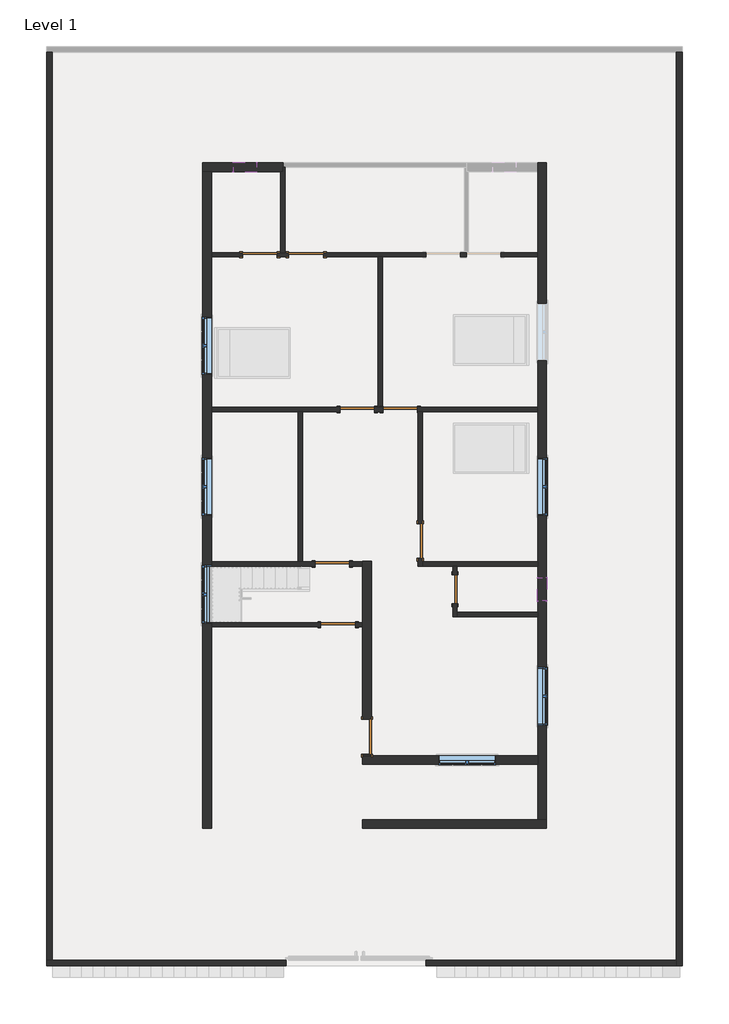
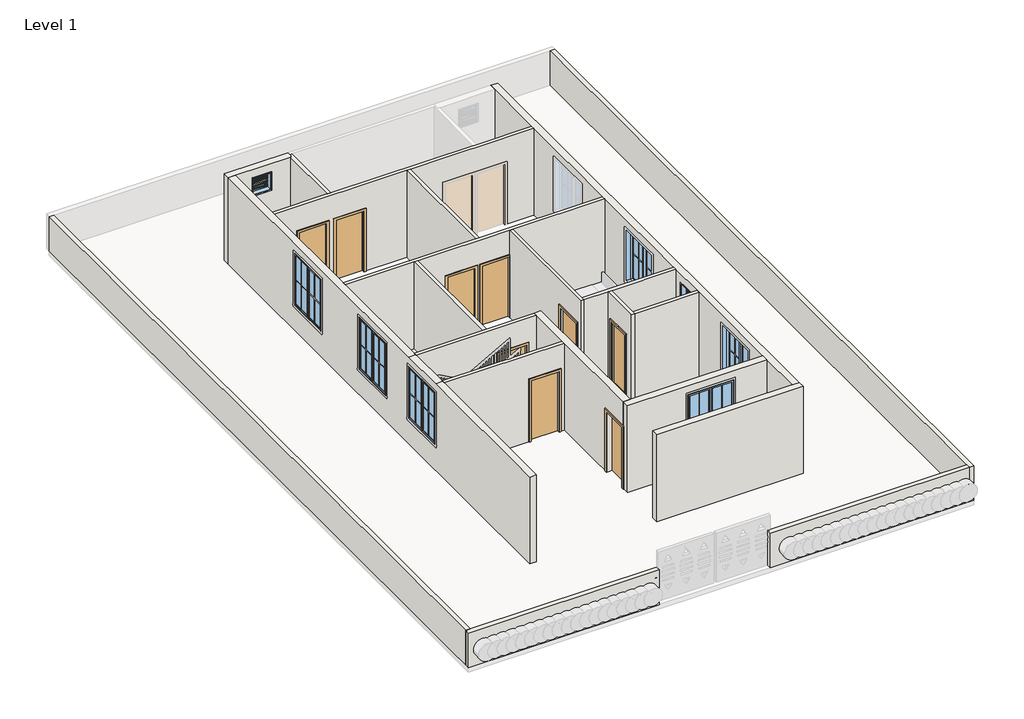
# One storey, part 1 of 3: 21 walls, 9 doors, 8 windows.
"""IFC4 building model written with IfcOpenShell, lengths in millimetres."""

from ifc_helpers import new_model, si_unit, frame, origin, origin_with_axes, place, context, project, spatial, polyline, outline, extrude, faceted_brep, transform, mapped, element, save
from components import door_78caadf7, single_flush_door_3_e5f9f3c4, single_flush_door_3_305aa2a5, single_flush_door_3_0ca8825f, window_casement_double_win_5_f93960c7, window_f2d8fef0

model = new_model("IFC4")

# Units and contexts
model_context = context("Model", 3, world=origin())
ifc_project = project(units=[si_unit("LENGTHUNIT", "METRE", prefix="MILLI")], contexts=[model_context])

# Site, building, storey
site = spatial("IfcSite", under=ifc_project)
building = spatial("IfcBuilding", under=site)
storey = spatial("IfcBuildingStorey", under=building, Name="Level 1", Elevation=0.0)

# Doors
placement = place(None, origin())
door_shape = door_78caadf7(model_context)
element("IfcDoor", 1, ObjectType="Single-Flush : DOOR 2'6\"", at=placement, inside=storey, context=model_context, shape_type="MappedRepresentation", body=[
    mapped(door_shape, transform((860.2379845, -2779.6065691, 0.0), x_axis=(0.0, 1.0, 0.0), y_axis=(-1.0, 0.0, 0.0), z_axis=(0.0, 0.0, 1.0))),
])
single_flush_door_3_shape = single_flush_door_3_e5f9f3c4(model_context)
element("IfcDoor", 2, ObjectType="Single-Flush : DOOR 3'", at=placement, inside=storey, context=model_context, shape_type="MappedRepresentation", body=[
    mapped(single_flush_door_3_shape, transform((-54.1620155, -1503.2565691, 0.0), x_axis=(0.0, -1.0, 0.0), y_axis=(1.0, 0.0, 0.0), z_axis=(0.0, 0.0, 1.0))),
])
element("IfcDoor", 3, ObjectType="Single-Flush : DOOR 3'", at=placement, inside=storey, context=model_context, shape_type="MappedRepresentation", body=[
    mapped(single_flush_door_3_shape, transform((-1717.8620155, 1963.8434309, 0.0), x_axis=(1.0, 0.0, 0.0), y_axis=(0.0, 1.0, 0.0), z_axis=(0.0, 0.0, 1.0))),
])
element("IfcDoor", 4, ObjectType="Single-Flush : DOOR 3'", at=placement, inside=storey, context=model_context, shape_type="MappedRepresentation", body=[
    mapped(single_flush_door_3_shape, transform((-2371.9120155, -2112.8565691, 0.0), x_axis=(1.0, 0.0, 0.0), y_axis=(0.0, 1.0, 0.0), z_axis=(0.0, 0.0, 1.0))),
])
element("IfcDoor", 5, ObjectType="Single-Flush : DOOR 3'", at=placement, inside=storey, context=model_context, shape_type="MappedRepresentation", body=[
    mapped(single_flush_door_3_shape, transform((-2219.5120155, -3713.0565691, 0.0), x_axis=(1.0, 0.0, 0.0), y_axis=(0.0, 1.0, 0.0), z_axis=(0.0, 0.0, 1.0))),
])
element("IfcDoor", 6, ObjectType="Single-Flush : DOOR 3'", at=placement, inside=storey, context=model_context, shape_type="MappedRepresentation", body=[
    mapped(single_flush_door_3_shape, transform((-4283.2620155, 6040.5434309, 0.0), x_axis=(1.0, 0.0, 0.0), y_axis=(0.0, 1.0, 0.0), z_axis=(0.0, 0.0, 1.0))),
])
single_flush_door_3_2_shape = single_flush_door_3_305aa2a5(model_context)
element("IfcDoor", 7, ObjectType="Single-Flush : DOOR 3'", at=placement, inside=storey, context=model_context, shape_type="MappedRepresentation", body=[
    mapped(single_flush_door_3_2_shape, transform((-581.2120155, 1963.8434309, 0.0), x_axis=(-1.0, 0.0, 0.0), y_axis=(0.0, -1.0, 0.0), z_axis=(0.0, 0.0, 1.0))),
])
element("IfcDoor", 8, ObjectType="Single-Flush : DOOR 3'", at=placement, inside=storey, context=model_context, shape_type="MappedRepresentation", body=[
    mapped(single_flush_door_3_2_shape, transform((-3064.0620155, 6040.5434309, 0.0), x_axis=(-1.0, 0.0, 0.0), y_axis=(0.0, -1.0, 0.0), z_axis=(0.0, 0.0, 1.0))),
])
single_flush_door_3_3_shape = single_flush_door_3_0ca8825f(model_context)
element("IfcDoor", 9, ObjectType="Single-Flush : DOOR 3'", at=placement, inside=storey, context=model_context, shape_type="MappedRepresentation", body=[
    mapped(single_flush_door_3_3_shape, transform((-1457.5120155, -6665.8065691, 0.0), x_axis=(0.0, -1.0, 0.0), y_axis=(1.0, 0.0, 0.0), z_axis=(0.0, 0.0, 1.0))),
])

# Walls
element("IfcWall", 10, ObjectType="CMD 6\"", at=placement, inside=storey, context=model_context, shape_type="Brep", body=[
    faceted_brep([(6701.4726148, 11374.8947978, 0.0), (6701.4726148, -12551.9052022, 0.0), (6701.4726148, -12704.3052022, 0.0), (6701.4726148, -12704.3052022, 1219.2), (6701.4726148, -12551.9052022, 1219.2), (6701.4726148, 11374.8947978, 1219.2), (6853.8726148, 11374.8947978, 0.0), (6853.8726148, 11374.8947978, 1219.2), (6853.8726148, -12704.3052022, 1219.2), (6853.8726148, -12704.3052022, 0.0)], [[[0, 1, 2, 3, 4, 5]], [[6, 7, 8, 9]], [[2, 1, 0, 6, 9]], [[5, 4, 3, 8, 7]], [[0, 5, 7, 6]], [[3, 2, 9, 8]]]),
])
element("IfcWall", 11, ObjectType="CMD 6\"", at=placement, inside=storey, context=model_context, shape_type="SweptSolid", body=[
    extrude(outline(polyline([(102.2665881, -12551.9052022), (6701.4726148, -12551.9052022), (6701.4726148, -12704.3052022), (102.2665881, -12704.3052022), (102.2665881, -12551.9052022)])), origin_with_axes(), (0.0, 0.0, 1.0), 1219.2),
])
element("IfcWall", 12, ObjectType="CMD 6\"", at=placement, inside=storey, context=model_context, shape_type="SweptSolid", body=[
    extrude(outline(polyline([(-9757.7273852, 11374.8947978), (-9757.7273852, -12551.9052022), (-9910.1273852, -12551.9052022), (-9910.1273852, 11374.8947978), (-9757.7273852, 11374.8947978)])), origin_with_axes(), (0.0, 0.0, 1.0), 1219.2),
])
element("IfcWall", 13, ObjectType="CMD 6\"", at=placement, inside=storey, context=model_context, shape_type="Brep", body=[
    faceted_brep([(-3585.5273852, -12551.9052022, 0.0), (-9757.7273852, -12551.9052022, 0.0), (-9910.1273852, -12551.9052022, 0.0), (-9910.1273852, -12551.9052022, 1219.2), (-9757.7273852, -12551.9052022, 1219.2), (-3585.5273852, -12551.9052022, 1219.2), (-3585.5273852, -12704.3052022, 0.0), (-3585.5273852, -12704.3052022, 1219.2), (-9910.1273852, -12704.3052022, 1219.2), (-9910.1273852, -12704.3052022, 0.0)], [[[0, 1, 2, 3, 4, 5]], [[6, 7, 8, 9]], [[2, 1, 0, 6, 9]], [[5, 4, 3, 8, 7]], [[0, 5, 7, 6]], [[3, 2, 9, 8]]]),
])
element("IfcWall", 14, ObjectType="WALL 4.5\"", at=placement, inside=storey, context=model_context, shape_type="SweptSolid", body=[
    extrude(outline(polyline([(-3730.8120155, 6097.6934309), (-3730.8120155, 8231.2934309), (-3673.6620155, 8231.2934309), (-3673.6620155, 8345.5934309), (-3616.5120155, 8345.5934309), (-3616.5120155, 6097.6934309), (-3730.8120155, 6097.6934309)])), origin_with_axes(), (0.0, 0.0, 1.0), 3048.0),
])
element("IfcWall", 15, ObjectType="WALL 4.5\"", at=placement, inside=storey, context=model_context, shape_type="Brep", body=[
    faceted_brep([(1165.0379845, 6097.6934309, 2133.6), (1165.0379845, 6097.6934309, 0.0), (1107.8879845, 6097.6934309, 0.0), (1012.6379845, 6097.6934309, 0.0), (1012.6379845, 6097.6934309, 2133.6), (98.2379845, 6097.6934309, 2133.6), (98.2379845, 6097.6934309, 0.0), (-2606.8620155, 6097.6934309, 0.0), (-2606.8620155, 6097.6934309, 2133.6), (-3521.2620155, 6097.6934309, 2133.6), (-3521.2620155, 6097.6934309, 0.0), (-3616.5120155, 6097.6934309, 0.0), (-3730.8120155, 6097.6934309, 0.0), (-3826.0620155, 6097.6934309, 0.0), (-3826.0620155, 6097.6934309, 2133.6), (-4740.4620155, 6097.6934309, 2133.6), (-4740.4620155, 6097.6934309, 0.0), (-5559.6120155, 6097.6934309, 0.0), (-5559.6120155, 6097.6934309, 3048.0), (-3730.8120155, 6097.6934309, 3048.0), (-3616.5120155, 6097.6934309, 3048.0), (1107.8879845, 6097.6934309, 3048.0), (1222.1879845, 6097.6934309, 3048.0), (3050.9879845, 6097.6934309, 3048.0), (3050.9879845, 6097.6934309, 0.0), (2079.4379845, 6097.6934309, 0.0), (2079.4379845, 6097.6934309, 2133.6), (1012.6379845, 5983.3934309, 0.0), (1165.0379845, 5983.3934309, 0.0), (1165.0379845, 5983.3934309, 2133.6), (2079.4379845, 5983.3934309, 2133.6), (2079.4379845, 5983.3934309, 0.0), (3050.9879845, 5983.3934309, 0.0), (3050.9879845, 5983.3934309, 3048.0), (-1051.1120155, 5983.3934309, 3048.0), (-1165.4120155, 5983.3934309, 3048.0), (-5559.6120155, 5983.3934309, 3048.0), (-5559.6120155, 5983.3934309, 0.0), (-4740.4620155, 5983.3934309, 0.0), (-4740.4620155, 5983.3934309, 2133.6), (-3826.0620155, 5983.3934309, 2133.6), (-3826.0620155, 5983.3934309, 0.0), (-3521.2620155, 5983.3934309, 0.0), (-3521.2620155, 5983.3934309, 2133.6), (-2606.8620155, 5983.3934309, 2133.6), (-2606.8620155, 5983.3934309, 0.0), (-1165.4120155, 5983.3934309, 0.0), (-1051.1120155, 5983.3934309, 0.0), (98.2379845, 5983.3934309, 0.0), (98.2379845, 5983.3934309, 2133.6), (1012.6379845, 5983.3934309, 2133.6)], [[[0, 1, 2, 3, 4, 5, 6, 7, 8, 9, 10, 11, 12, 13, 14, 15, 16, 17, 18, 19, 20, 21, 22, 23, 24, 25, 26]], [[27, 28, 29, 30, 31, 32, 33, 34, 35, 36, 37, 38, 39, 40, 41, 42, 43, 44, 45, 46, 47, 48, 49, 50]], [[38, 37, 17, 16]], [[13, 12, 11, 10, 42, 41]], [[48, 47, 46, 45, 7, 6]], [[25, 24, 32, 31]], [[3, 2, 1, 28, 27]], [[18, 17, 37, 36]], [[24, 23, 33, 32]], [[14, 13, 41, 40]], [[15, 14, 40, 39]], [[16, 15, 39, 38]], [[43, 42, 10, 9]], [[44, 43, 9, 8]], [[45, 44, 8, 7]], [[4, 3, 27, 50]], [[5, 4, 50, 49]], [[6, 5, 49, 48]], [[29, 28, 1, 0]], [[30, 29, 0, 26]], [[31, 30, 26, 25]], [[23, 22, 21, 20, 19, 18, 36, 35, 34, 33]]]),
])
element("IfcWall", 16, ObjectType="WALL 4.5\"", at=placement, inside=storey, context=model_context, shape_type="SweptSolid", body=[
    extrude(outline(polyline([(-1165.4120155, 2020.9934309), (-1165.4120155, 5983.3934309), (-1051.1120155, 5983.3934309), (-1051.1120155, 2020.9934309), (-1165.4120155, 2020.9934309)])), origin_with_axes(), (0.0, 0.0, 1.0), 3048.0),
])
element("IfcWall", 17, ObjectType="WALL 4.5\"", at=placement, inside=storey, context=model_context, shape_type="Brep", body=[
    faceted_brep([(-1260.6620155, 1906.6934309, 2133.6), (-1260.6620155, 1906.6934309, 0.0), (-1038.4120155, 1906.6934309, 0.0), (-1038.4120155, 1906.6934309, 2133.6), (-124.0120155, 1906.6934309, 2133.6), (-124.0120155, 1906.6934309, 0.0), (-111.3120155, 1906.6934309, 0.0), (2.9879845, 1906.6934309, 0.0), (3050.9879845, 1906.6934309, 0.0), (3050.9879845, 1906.6934309, 3048.0), (2.9879845, 1906.6934309, 3048.0), (-111.3120155, 1906.6934309, 3048.0), (-3159.3120155, 1906.6934309, 3048.0), (-3273.6120155, 1906.6934309, 3048.0), (-5559.6120155, 1906.6934309, 3048.0), (-5559.6120155, 1906.6934309, 0.0), (-3273.6120155, 1906.6934309, 0.0), (-3159.3120155, 1906.6934309, 0.0), (-2175.0620155, 1906.6934309, 0.0), (-2175.0620155, 1906.6934309, 2133.6), (-1038.4120155, 2020.9934309, 0.0), (-1051.1120155, 2020.9934309, 0.0), (-1165.4120155, 2020.9934309, 0.0), (-1260.6620155, 2020.9934309, 0.0), (-1260.6620155, 2020.9934309, 2133.6), (-2175.0620155, 2020.9934309, 2133.6), (-2175.0620155, 2020.9934309, 0.0), (-5559.6120155, 2020.9934309, 0.0), (-5559.6120155, 2020.9934309, 3048.0), (-1165.4120155, 2020.9934309, 3048.0), (-1051.1120155, 2020.9934309, 3048.0), (3050.9879845, 2020.9934309, 3048.0), (3050.9879845, 2020.9934309, 0.0), (-124.0120155, 2020.9934309, 0.0), (-124.0120155, 2020.9934309, 2133.6), (-1038.4120155, 2020.9934309, 2133.6)], [[[0, 1, 2, 3, 4, 5, 6, 7, 8, 9, 10, 11, 12, 13, 14, 15, 16, 17, 18, 19]], [[20, 21, 22, 23, 24, 25, 26, 27, 28, 29, 30, 31, 32, 33, 34, 35]], [[33, 32, 8, 7, 6, 5]], [[2, 1, 23, 22, 21, 20]], [[18, 17, 16, 15, 27, 26]], [[15, 14, 28, 27]], [[9, 8, 32, 31]], [[3, 2, 20, 35]], [[4, 3, 35, 34]], [[5, 4, 34, 33]], [[24, 23, 1, 0]], [[25, 24, 0, 19]], [[26, 25, 19, 18]], [[14, 13, 12, 11, 10, 9, 31, 30, 29, 28]]]),
])
element("IfcWall", 18, ObjectType="WALL 4.5\"", at=placement, inside=storey, context=model_context, shape_type="SweptSolid", body=[
    extrude(outline(polyline([(-3273.6120155, -2032.8465691), (-3273.6120155, 1906.6934309), (-3159.3120155, 1906.6934309), (-3159.3120155, -2032.8465691), (-3273.6120155, -2032.8465691)])), origin_with_axes(), (0.0, 0.0, 1.0), 3048.0),
])
element("IfcWall", 19, ObjectType="WALL 4.5\"", at=placement, inside=storey, context=model_context, shape_type="SweptSolid", body=[
    extrude(outline(polyline([(2133.6, -1914.7120155), (0.0, -1914.7120155), (0.0, -1571.8120155), (3048.0, -1571.8120155), (3048.0, -5559.6120155), (0.0, -5559.6120155), (0.0, -2829.1120155), (2133.6, -2829.1120155), (2133.6, -1914.7120155)])), frame((0.0, -2170.0065691, 0.0), z_axis=(0.0, 1.0, 0.0), x_axis=(0.0, 0.0, 1.0)), (0.0, 0.0, 1.0), 114.3),
])
element("IfcWall", 20, ObjectType="WALL 4.5\"", at=placement, inside=storey, context=model_context, shape_type="SweptSolid", body=[
    extrude(outline(polyline([(2133.6, -1762.3120155), (0.0, -1762.3120155), (0.0, -1571.8120155), (3048.0, -1571.8120155), (3048.0, -5559.6120155), (0.0, -5559.6120155), (0.0, -2676.7120155), (2133.6, -2676.7120155), (2133.6, -1762.3120155)])), frame((0.0, -3770.2065691, 0.0), z_axis=(0.0, 1.0, 0.0), x_axis=(0.0, 0.0, 1.0)), (0.0, 0.0, 1.0), 114.3),
])
element("IfcWall", 21, ObjectType="WALL 4.5\"", at=placement, inside=storey, context=model_context, shape_type="Brep", body=[
    faceted_brep([(-111.3120155, -1960.4565691, 2133.6), (-111.3120155, -1960.4565691, 0.0), (-111.3120155, -2170.0065691, 0.0), (-111.3120155, -2170.0065691, 3048.0), (-111.3120155, 1906.6934309, 3048.0), (-111.3120155, 1906.6934309, 0.0), (-111.3120155, -1046.0565691, 0.0), (-111.3120155, -1046.0565691, 2133.6), (2.9879845, -2170.0065691, 0.0), (2.9879845, -2055.7065691, 0.0), (2.9879845, -1960.4565691, 0.0), (2.9879845, -1960.4565691, 2133.6), (2.9879845, -1046.0565691, 2133.6), (2.9879845, -1046.0565691, 0.0), (2.9879845, 1906.6934309, 0.0), (2.9879845, 1906.6934309, 3048.0), (2.9879845, -2055.7065691, 3048.0), (2.9879845, -2170.0065691, 3048.0)], [[[0, 1, 2, 3, 4, 5, 6, 7]], [[8, 9, 10, 11, 12, 13, 14, 15, 16, 17]], [[6, 5, 14, 13]], [[2, 1, 10, 9, 8]], [[5, 4, 15, 14]], [[3, 2, 8, 17]], [[11, 10, 1, 0]], [[12, 11, 0, 7]], [[13, 12, 7, 6]], [[4, 3, 17, 16, 15]]]),
])
element("IfcWall", 22, ObjectType="WALL 4.5\"", at=placement, inside=storey, context=model_context, shape_type="Brep", body=[
    faceted_brep([(2.9879845, -2170.0065691, 0.0), (803.0879845, -2170.0065691, 0.0), (917.3879845, -2170.0065691, 0.0), (3050.9879845, -2170.0065691, 0.0), (3050.9879845, -2170.0065691, 3048.0), (917.3879845, -2170.0065691, 3048.0), (803.0879845, -2170.0065691, 3048.0), (2.9879845, -2170.0065691, 3048.0), (2.9879845, -2055.7065691, 0.0), (2.9879845, -2055.7065691, 3048.0), (3050.9879845, -2055.7065691, 3048.0), (3050.9879845, -2055.7065691, 0.0)], [[[0, 1, 2, 3, 4, 5, 6, 7]], [[8, 9, 10, 11]], [[3, 2, 1, 0, 8, 11]], [[0, 7, 9, 8]], [[4, 3, 11, 10]], [[7, 6, 5, 4, 10, 9]]]),
])
element("IfcWall", 23, ObjectType="WALL 4.5\"", at=placement, inside=storey, context=model_context, shape_type="Brep", body=[
    faceted_brep([(803.0879845, -2170.0065691, 0.0), (803.0879845, -2398.6065691, 0.0), (803.0879845, -2398.6065691, 2133.6), (803.0879845, -3160.6065691, 2133.6), (803.0879845, -3160.6065691, 0.0), (803.0879845, -3503.5065691, 0.0), (803.0879845, -3503.5065691, 3048.0), (803.0879845, -2170.0065691, 3048.0), (917.3879845, -2398.6065691, 2133.6), (917.3879845, -2398.6065691, 0.0), (917.3879845, -2170.0065691, 0.0), (917.3879845, -2170.0065691, 3048.0), (917.3879845, -3389.2065691, 3048.0), (917.3879845, -3503.5065691, 3048.0), (917.3879845, -3503.5065691, 0.0), (917.3879845, -3389.2065691, 0.0), (917.3879845, -3160.6065691, 0.0), (917.3879845, -3160.6065691, 2133.6)], [[[0, 1, 2, 3, 4, 5, 6, 7]], [[8, 9, 10, 11, 12, 13, 14, 15, 16, 17]], [[10, 9, 1, 0]], [[16, 15, 14, 5, 4]], [[0, 7, 11, 10]], [[6, 5, 14, 13]], [[2, 1, 9, 8]], [[3, 2, 8, 17]], [[4, 3, 17, 16]], [[7, 6, 13, 12, 11]]]),
])
element("IfcWall", 24, ObjectType="WALL 4.5\"", at=placement, inside=storey, context=model_context, shape_type="SweptSolid", body=[
    extrude(outline(polyline([(917.3879845, -3389.2065691), (3050.9879845, -3389.2065691), (3050.9879845, -3503.5065691), (917.3879845, -3503.5065691), (917.3879845, -3389.2065691)])), origin_with_axes(), (0.0, 0.0, 1.0), 3048.0),
])
element("IfcWall", 25, ObjectType="WALL 9\"", at=placement, inside=storey, context=model_context, shape_type="Brep", body=[
    faceted_brep([(-3673.6620155, 8459.8934309, 0.0), (-5788.2120155, 8459.8934309, 0.0), (-5788.2120155, 8459.8934309, 3048.0), (-3673.6620155, 8459.8934309, 3048.0), (-4978.5870155, 8459.8934309, 2743.2), (-4978.5870155, 8459.8934309, 2133.6), (-4368.9870155, 8459.8934309, 2133.6), (-4368.9870155, 8459.8934309, 2743.2), (-3673.6620155, 8231.2934309, 0.0), (-3673.6620155, 8231.2934309, 3048.0), (-3730.8120155, 8231.2934309, 3048.0), (-5559.6120155, 8231.2934309, 3048.0), (-5788.2120155, 8231.2934309, 3048.0), (-5788.2120155, 8231.2934309, 0.0), (-5559.6120155, 8231.2934309, 0.0), (-3730.8120155, 8231.2934309, 0.0), (-4978.5870155, 8231.2934309, 2743.2), (-4368.9870155, 8231.2934309, 2743.2), (-4368.9870155, 8231.2934309, 2133.6), (-4978.5870155, 8231.2934309, 2133.6), (-3673.6620155, 8345.5934309, 0.0), (-3673.6620155, 8345.5934309, 3048.0)], [[[0, 1, 2, 3], [4, 5, 6, 7]], [[8, 9, 10, 11, 12, 13, 14, 15], [16, 17, 18, 19]], [[1, 0, 20, 8, 15, 14, 13]], [[0, 3, 21, 9, 8, 20]], [[2, 1, 13, 12]], [[5, 4, 16, 19]], [[6, 5, 19, 18]], [[7, 6, 18, 17]], [[4, 7, 17, 16]], [[3, 2, 12, 11, 10, 9, 21]]]),
])
element("IfcWall", 26, ObjectType="WALL 9\"", at=placement, inside=storey, context=model_context, shape_type="Brep", body=[
    faceted_brep([(-5788.2120155, 8231.2934309, 0.0), (-5788.2120155, -9078.8065691, 0.0), (-5788.2120155, -9078.8065691, 3048.0), (-5788.2120155, -3674.9565691, 3048.0), (-5788.2120155, -2150.9565691, 3048.0), (-5788.2120155, 8231.2934309, 3048.0), (-5788.2120155, 4402.2434309, 2743.2), (-5788.2120155, 2878.2434309, 2743.2), (-5788.2120155, 2878.2434309, 914.4), (-5788.2120155, 4402.2434309, 914.4), (-5788.2120155, -2150.9565691, 2743.2), (-5788.2120155, -3674.9565691, 2743.2), (-5788.2120155, -3674.9565691, 914.4), (-5788.2120155, -2150.9565691, 914.4), (-5788.2120155, 687.4934309, 2743.2), (-5788.2120155, -836.5065691, 2743.2), (-5788.2120155, -836.5065691, 914.4), (-5788.2120155, 687.4934309, 914.4), (-5559.6120155, 8231.2934309, 0.0), (-5559.6120155, 8231.2934309, 3048.0), (-5559.6120155, 6097.6934309, 3048.0), (-5559.6120155, 5983.3934309, 3048.0), (-5559.6120155, 2020.9934309, 3048.0), (-5559.6120155, 1906.6934309, 3048.0), (-5559.6120155, -2055.7065691, 3048.0), (-5559.6120155, -2150.9565691, 3048.0), (-5559.6120155, -2170.0065691, 3048.0), (-5559.6120155, -3655.9065691, 3048.0), (-5559.6120155, -3674.9565691, 3048.0), (-5559.6120155, -3770.2065691, 3048.0), (-5559.6120155, -9078.8065691, 3048.0), (-5559.6120155, -9078.8065691, 0.0), (-5559.6120155, -3770.2065691, 0.0), (-5559.6120155, -3655.9065691, 0.0), (-5559.6120155, -2170.0065691, 0.0), (-5559.6120155, -2055.7065691, 0.0), (-5559.6120155, 1906.6934309, 0.0), (-5559.6120155, 2020.9934309, 0.0), (-5559.6120155, 5983.3934309, 0.0), (-5559.6120155, 6097.6934309, 0.0), (-5559.6120155, 4402.2434309, 2743.2), (-5559.6120155, 4402.2434309, 914.4), (-5559.6120155, 2878.2434309, 914.4), (-5559.6120155, 2878.2434309, 2743.2), (-5559.6120155, -2150.9565691, 2743.2), (-5559.6120155, -2150.9565691, 914.4), (-5559.6120155, -3674.9565691, 914.4), (-5559.6120155, -3674.9565691, 2743.2), (-5559.6120155, 687.4934309, 2743.2), (-5559.6120155, 687.4934309, 914.4), (-5559.6120155, -836.5065691, 914.4), (-5559.6120155, -836.5065691, 2743.2)], [[[0, 1, 2, 3, 4, 5], [6, 7, 8, 9], [10, 11, 12, 13], [14, 15, 16, 17]], [[18, 19, 20, 21, 22, 23, 24, 25, 26, 27, 28, 29, 30, 31, 32, 33, 34, 35, 36, 37, 38, 39], [40, 41, 42, 43], [44, 45, 46, 47], [48, 49, 50, 51]], [[1, 0, 18, 39, 38, 37, 36, 35, 34, 33, 32, 31]], [[2, 1, 31, 30]], [[0, 5, 19, 18]], [[41, 40, 6, 9]], [[42, 41, 9, 8]], [[43, 42, 8, 7]], [[40, 43, 7, 6]], [[45, 44, 10, 13]], [[46, 45, 13, 12]], [[47, 46, 12, 11]], [[44, 47, 11, 10]], [[49, 48, 14, 17]], [[50, 49, 17, 16]], [[51, 50, 16, 15]], [[48, 51, 15, 14]], [[4, 3, 28, 27, 26, 25]], [[3, 2, 30, 29, 28]], [[5, 4, 25, 24, 23, 22, 21, 20, 19]]]),
])
element("IfcWall", 27, ObjectType="WALL 9\"", at=placement, inside=storey, context=model_context, shape_type="Brep", body=[
    faceted_brep([(-1571.8120155, -9078.8065691, 0.0), (3279.5879845, -9078.8065691, 0.0), (3279.5879845, -9078.8065691, 3048.0), (-1571.8120155, -9078.8065691, 3048.0), (-1571.8120155, -8850.2065691, 0.0), (-1571.8120155, -8850.2065691, 3048.0), (3050.9879845, -8850.2065691, 3048.0), (3279.5879845, -8850.2065691, 3048.0), (3279.5879845, -8850.2065691, 0.0), (3050.9879845, -8850.2065691, 0.0)], [[[0, 1, 2, 3]], [[4, 5, 6, 7, 8, 9]], [[1, 0, 4, 9, 8]], [[0, 3, 5, 4]], [[2, 1, 8, 7]], [[3, 2, 7, 6, 5]]]),
])
element("IfcWall", 28, ObjectType="WALL 9\"", at=placement, inside=storey, context=model_context, shape_type="Brep", body=[
    faceted_brep([(3279.5879845, -8850.2065691, 0.0), (3279.5879845, 8459.8934309, 0.0), (3279.5879845, 8459.8934309, 3048.0), (3279.5879845, -8850.2065691, 3048.0), (3279.5879845, 3240.1934309, 2743.2), (3279.5879845, 4764.1934309, 2743.2), (3279.5879845, 4764.1934309, 914.4), (3279.5879845, 3240.1934309, 914.4), (3279.5879845, -836.5065691, 2743.2), (3279.5879845, 687.4934309, 2743.2), (3279.5879845, 687.4934309, 914.4), (3279.5879845, -836.5065691, 914.4), (3279.5879845, -6361.0065691, 2743.2), (3279.5879845, -4837.0065691, 2743.2), (3279.5879845, -4837.0065691, 914.4), (3279.5879845, -6361.0065691, 914.4), (3279.5879845, -2474.8065691, 2743.2), (3279.5879845, -2474.8065691, 2133.6), (3279.5879845, -3084.4065691, 2133.6), (3279.5879845, -3084.4065691, 2743.2), (3050.9879845, -8850.2065691, 0.0), (3050.9879845, -8850.2065691, 3048.0), (3050.9879845, -7389.7065691, 3048.0), (3050.9879845, -7161.1065691, 3048.0), (3050.9879845, -3503.5065691, 3048.0), (3050.9879845, -3389.2065691, 3048.0), (3050.9879845, -2170.0065691, 3048.0), (3050.9879845, -2055.7065691, 3048.0), (3050.9879845, 1906.6934309, 3048.0), (3050.9879845, 2020.9934309, 3048.0), (3050.9879845, 5983.3934309, 3048.0), (3050.9879845, 6097.6934309, 3048.0), (3050.9879845, 8231.2934309, 3048.0), (3050.9879845, 8459.8934309, 3048.0), (3050.9879845, 8459.8934309, 0.0), (3050.9879845, 8231.2934309, 0.0), (3050.9879845, 6097.6934309, 0.0), (3050.9879845, 5983.3934309, 0.0), (3050.9879845, 2020.9934309, 0.0), (3050.9879845, 1906.6934309, 0.0), (3050.9879845, -2055.7065691, 0.0), (3050.9879845, -2170.0065691, 0.0), (3050.9879845, -3389.2065691, 0.0), (3050.9879845, -3503.5065691, 0.0), (3050.9879845, -7161.1065691, 0.0), (3050.9879845, -7389.7065691, 0.0), (3050.9879845, 3240.1934309, 2743.2), (3050.9879845, 3240.1934309, 914.4), (3050.9879845, 4764.1934309, 914.4), (3050.9879845, 4764.1934309, 2743.2), (3050.9879845, -836.5065691, 2743.2), (3050.9879845, -836.5065691, 914.4), (3050.9879845, 687.4934309, 914.4), (3050.9879845, 687.4934309, 2743.2), (3050.9879845, -6361.0065691, 2743.2), (3050.9879845, -6361.0065691, 914.4), (3050.9879845, -4837.0065691, 914.4), (3050.9879845, -4837.0065691, 2743.2), (3050.9879845, -2474.8065691, 2743.2), (3050.9879845, -3084.4065691, 2743.2), (3050.9879845, -3084.4065691, 2133.6), (3050.9879845, -2474.8065691, 2133.6)], [[[0, 1, 2, 3], [4, 5, 6, 7], [8, 9, 10, 11], [12, 13, 14, 15], [16, 17, 18, 19]], [[20, 21, 22, 23, 24, 25, 26, 27, 28, 29, 30, 31, 32, 33, 34, 35, 36, 37, 38, 39, 40, 41, 42, 43, 44, 45], [46, 47, 48, 49], [50, 51, 52, 53], [54, 55, 56, 57], [58, 59, 60, 61]], [[1, 0, 20, 45, 44, 43, 42, 41, 40, 39, 38, 37, 36, 35, 34]], [[0, 3, 21, 20]], [[2, 1, 34, 33]], [[47, 46, 4, 7]], [[48, 47, 7, 6]], [[49, 48, 6, 5]], [[46, 49, 5, 4]], [[51, 50, 8, 11]], [[52, 51, 11, 10]], [[53, 52, 10, 9]], [[50, 53, 9, 8]], [[55, 54, 12, 15]], [[56, 55, 15, 14]], [[57, 56, 14, 13]], [[54, 57, 13, 12]], [[17, 16, 58, 61]], [[18, 17, 61, 60]], [[19, 18, 60, 59]], [[16, 19, 59, 58]], [[3, 2, 33, 32, 31, 30, 29, 28, 27, 26, 25, 24, 23, 22, 21]]]),
])
element("IfcWall", 29, ObjectType="WALL 9\"", at=placement, inside=storey, context=model_context, shape_type="Brep", body=[
    faceted_brep([(3050.9879845, -7161.1065691, 0.0), (-1343.2120155, -7161.1065691, 0.0), (-1571.8120155, -7161.1065691, 0.0), (-1571.8120155, -7161.1065691, 3048.0), (-1343.2120155, -7161.1065691, 3048.0), (3050.9879845, -7161.1065691, 3048.0), (422.0879845, -7161.1065691, 2743.2), (422.0879845, -7161.1065691, 914.4), (1946.0879845, -7161.1065691, 914.4), (1946.0879845, -7161.1065691, 2743.2), (3050.9879845, -7389.7065691, 0.0), (3050.9879845, -7389.7065691, 3048.0), (-1571.8120155, -7389.7065691, 3048.0), (-1571.8120155, -7389.7065691, 0.0), (422.0879845, -7389.7065691, 2743.2), (1946.0879845, -7389.7065691, 2743.2), (1946.0879845, -7389.7065691, 914.4), (422.0879845, -7389.7065691, 914.4)], [[[0, 1, 2, 3, 4, 5], [6, 7, 8, 9]], [[10, 11, 12, 13], [14, 15, 16, 17]], [[2, 1, 0, 10, 13]], [[0, 5, 11, 10]], [[3, 2, 13, 12]], [[7, 6, 14, 17]], [[8, 7, 17, 16]], [[9, 8, 16, 15]], [[6, 9, 15, 14]], [[5, 4, 3, 12, 11]]]),
])
element("IfcWall", 30, ObjectType="WALL 9\"", at=placement, inside=storey, context=model_context, shape_type="Brep", body=[
    faceted_brep([(-1343.2120155, -7161.1065691, 0.0), (-1343.2120155, -7123.0065691, 0.0), (-1343.2120155, -7123.0065691, 2133.6), (-1343.2120155, -6208.6065691, 2133.6), (-1343.2120155, -6208.6065691, 0.0), (-1343.2120155, -2032.8465691, 0.0), (-1343.2120155, -2032.8465691, 3048.0), (-1343.2120155, -7161.1065691, 3048.0), (-1571.8120155, -7123.0065691, 2133.6), (-1571.8120155, -7123.0065691, 0.0), (-1571.8120155, -7161.1065691, 0.0), (-1571.8120155, -7161.1065691, 3048.0), (-1571.8120155, -3770.2065691, 3048.0), (-1571.8120155, -3655.9065691, 3048.0), (-1571.8120155, -2170.0065691, 3048.0), (-1571.8120155, -2055.7065691, 3048.0), (-1571.8120155, -2032.8465691, 3048.0), (-1571.8120155, -2032.8465691, 0.0), (-1571.8120155, -2055.7065691, 0.0), (-1571.8120155, -2170.0065691, 0.0), (-1571.8120155, -3655.9065691, 0.0), (-1571.8120155, -3770.2065691, 0.0), (-1571.8120155, -6208.6065691, 0.0), (-1571.8120155, -6208.6065691, 2133.6)], [[[0, 1, 2, 3, 4, 5, 6, 7]], [[8, 9, 10, 11, 12, 13, 14, 15, 16, 17, 18, 19, 20, 21, 22, 23]], [[10, 9, 1, 0]], [[22, 21, 20, 19, 18, 17, 5, 4]], [[6, 5, 17, 16]], [[0, 7, 11, 10]], [[2, 1, 9, 8]], [[3, 2, 8, 23]], [[4, 3, 23, 22]], [[7, 6, 16, 15, 14, 13, 12, 11]]]),
])

# Windows
window_casement_double_win_5_shape = window_casement_double_win_5_f93960c7(model_context)
element("IfcWindow", 31, ObjectType="Window-Casement-Double : WIN 5'", at=placement, inside=storey, context=model_context, shape_type="MappedRepresentation", body=[
    mapped(window_casement_double_win_5_shape, transform((-5673.9120155, 3640.2434309, 0.0), x_axis=(0.0, 1.0, 0.0), y_axis=(-1.0, 0.0, 0.0), z_axis=(0.0, 0.0, 1.0))),
])
element("IfcWindow", 32, ObjectType="Window-Casement-Double : WIN 5'", at=placement, inside=storey, context=model_context, shape_type="MappedRepresentation", body=[
    mapped(window_casement_double_win_5_shape, transform((3165.2879845, -74.5065691, 0.0), x_axis=(0.0, -1.0, 0.0), y_axis=(1.0, 0.0, 0.0), z_axis=(0.0, 0.0, 1.0))),
])
element("IfcWindow", 33, ObjectType="Window-Casement-Double : WIN 5'", at=placement, inside=storey, context=model_context, shape_type="MappedRepresentation", body=[
    mapped(window_casement_double_win_5_shape, transform((3165.2879845, -5599.0065691, 0.0), x_axis=(0.0, -1.0, 0.0), y_axis=(1.0, 0.0, 0.0), z_axis=(0.0, 0.0, 1.0))),
])
element("IfcWindow", 34, ObjectType="Window-Casement-Double : WIN 5'", at=placement, inside=storey, context=model_context, shape_type="MappedRepresentation", body=[
    mapped(window_casement_double_win_5_shape, transform((1184.0879845, -7275.4065691, 0.0), x_axis=(-1.0, 0.0, 0.0), y_axis=(0.0, -1.0, 0.0), z_axis=(0.0, 0.0, 1.0))),
])
element("IfcWindow", 35, ObjectType="Window-Casement-Double : WIN 5'", at=placement, inside=storey, context=model_context, shape_type="MappedRepresentation", body=[
    mapped(window_casement_double_win_5_shape, transform((-5673.9120155, -2912.9565691, 0.0), x_axis=(0.0, 1.0, 0.0), y_axis=(-1.0, 0.0, 0.0), z_axis=(0.0, 0.0, 1.0))),
])
element("IfcWindow", 36, ObjectType="Window-Casement-Double : WIN 5'", at=placement, inside=storey, context=model_context, shape_type="MappedRepresentation", body=[
    mapped(window_casement_double_win_5_shape, transform((-5673.9120155, -74.5065691, 0.0), x_axis=(0.0, 1.0, 0.0), y_axis=(-1.0, 0.0, 0.0), z_axis=(0.0, 0.0, 1.0))),
])
window_shape = window_f2d8fef0(model_context)
element("IfcWindow", 37, ObjectType="Window-Louvers : 24\" x 24\"", at=placement, inside=storey, context=model_context, shape_type="MappedRepresentation", body=[
    mapped(window_shape, transform((-4673.7870155, 8351.9434309, 1219.2), x_axis=(1.0, 0.0, 0.0), y_axis=(0.0, 1.0, 0.0), z_axis=(0.0, 0.0, 1.0))),
])
element("IfcWindow", 38, ObjectType="Window-Louvers : 24\" x 24\"", at=placement, inside=storey, context=model_context, shape_type="MappedRepresentation", body=[
    mapped(window_shape, transform((3171.6379845, -2779.6065691, 1219.2), x_axis=(0.0, -1.0, 0.0), y_axis=(1.0, 0.0, 0.0), z_axis=(0.0, 0.0, 1.0))),
])

save(model, "model.ifc")

# Revit data of these elements
# Type "Single-Flush : DOOR 2'6\""
#   Type Mark = "10"
#   Construction Type Id = "MDOOR"
#   Assembly Code = "C1020"
#   Analytic Construction = "Metal"
#   Thickness = 0' - 2"
#   Heat Transfer Coefficient (U) = 0.651978 BTU/(h·ft²·°F)
#   Height = 7' - 0"
#   Trim Projection Ext = 0' - 1"
#   Trim Projection Int = 0' - 1"
#   Trim Width = 0' - 3"
#   Width = 2' - 6"
#   Define Thermal Properties by = 1
#   Door Material = Door - Panel
#   Frame Material = Door - Frame
#   Visual Light Transmittance = 0
#   Solar Heat Gain Coefficient = 0
#   Function = (empty or 0)
#   Wall Closure = (empty or 0)
# Type "Single-Flush : DOOR 3'"
#   Type Mark = "9"
#   Construction Type Id = "MDOOR"
#   Assembly Code = "C1020"
#   Analytic Construction = "Metal"
#   Thickness = 0' - 2"
#   Heat Transfer Coefficient (U) = 0.651978 BTU/(h·ft²·°F)
#   Height = 7' - 0"
#   Trim Projection Ext = 0' - 1"
#   Trim Projection Int = 0' - 1"
#   Trim Width = 0' - 3"
#   Width = 3' - 0"
#   Define Thermal Properties by = 1
#   Door Material = Door - Panel
#   Frame Material = Door - Frame
#   Visual Light Transmittance = 0
#   Solar Heat Gain Coefficient = 0
#   Function = (empty or 0)
#   Wall Closure = (empty or 0)
# Type "CMD 6\""
#   Assembly Code = "B2010"
#   Layers, outside or top first: 0' - 6" no material (function 1)
# Type "WALL 4.5\""
#   Assembly Code = "B2010"
#   Layers, outside or top first: 0' - 4 1/2" no material (function 1)
# Type "WALL 9\""
#   Assembly Code = "B2010"
#   Layers, outside or top first: 0' - 9" no material (function 1)
# Type "Window-Casement-Double : WIN 5'"
#   Type Mark = "18"
#   Fire Rating = "0.5h"
#   Assembly Code = "B2020100"
#   Analytic Construction = "Double glazing - domestic"
#   Frame Extension [instance default] = 0' - 0 1/4"
#   Window Inset [instance default] = 0' - 0"
#   Wall Thickness [instance default] = 0' - 6"
#   Interior Wall Closure [instance default] = 0' - 2 1/4"
#   Half Width = 2' - 6"
#   Visual Light Transmittance = 0.81
#   Thermal Resistance (R) = 1.8146 (h·ft²·°F)/BTU
#   Solar Heat Gain Coefficient = 0.76
#   Rough Width = 5' - 0 1/2"
#   Rough Height = 6' - 0 1/2"
#   Height = 6' - 0"
#   Heat Transfer Coefficient (U) = 0.5511 BTU/(h·ft²·°F)
#   Exterior Wall Closure [instance default] = 0' - 1 1/4"
#   Extension Jamb [instance default] = 0' - 2 1/4"
#   Default Sill Height = 3' - 0"
#   Width = 5' - 0"
#   Muntin Visibility = yes
#   Interior Trim Visibility [instance default] = yes
#   Exterior Trim Visibility [instance default] = yes
#   Extension Jamb Visibility [instance default] = yes
#   Interior Trim Material = Wood - Stained
#   Muntin Pattern = Muntin Pattern_2x2 : Muntin Pattern_2x2
#   Interior Trim = Trim-Window-Interior-Flat : Picture Frame
#   Interior Frame Material = Wood - Stained
#   Glass Panel Material = Glass
#   Exterior Trim Material = Clad - White
#   Exterior Trim = Trim-Window-Exterior-Flat : with Sill
#   Exterior Frame Material = Clad - White
#   Wall Closure = (empty or 0)
# Type "Window-Louvers : 24\" x 24\""
#   Type Mark = "19"
#   Construction Type Id = "GSP4R"
#   Assembly Code = "B20"
#   Analytic Construction = "1/8 in Pilkington single glazing"
#   Visual Light Transmittance = 0.9
#   Thermal Resistance (R) = 1.53941 (h·ft²·°F)/BTU
#   Solar Heat Gain Coefficient = 0.78
#   Max Height = 1' - 11.74264"
#   Height = 2' - 0"
#   Heat Transfer Coefficient (U) = 0.6496 BTU/(h·ft²·°F)
#   Blade Width [instance default] = 1' - 10 1/2"
#   Blade Vertical Thickness = 0' - 0.35355"
#   Blade Thickness = 0' - 0 1/4"
#   Blade Spacing = 0' - 1 1/2"
#   Blade Height = 0' - 1.85355"
#   Blade Depth = 0' - 3"
#   Blade Angle = 45.00°
#   Default Sill Height = 3' - 0"
#   Trim Projection_Exterior = 0' - 0 1/2"
#   Trim Projection_Interior = 0' - 0 1/2"
#   Trim Width_Exterior = 0' - 1 1/2"
#   Trim Width_Interior = 0' - 1 1/2"
#   Width = 2' - 0"
#   Max Blade Count = 12
#   Define Thermal Properties by = 1
#   Blade Count = 12
#   Frame Material = Birch
#   Louver Material = Birch
#   Trim Exterior Material = Birch
#   Trim Interior Material = Birch
#   Wall Closure = (empty or 0)
# Element 1 (IfcDoor, "Single-Flush : DOOR 2'6\"")
#   Phase Created = New Construction
#   Materials on its faces: "Door - Frame", "Door - Panel"
# Elements 2, 3, 4, 5, 6, 7, 8, 9 (IfcDoor, "Single-Flush : DOOR 3'")
#   Phase Created = New Construction
#   Materials on its faces: "Door - Frame", "Door - Panel"
# Elements 10, 13 (IfcWall, "CMD 6\"")
#   Top Offset = 0' - 0"
#   Base Offset = 0' - 0"
#   Unconnected Height = 4' - 0"
#   wall height = 4' - 0"
#   Phase Created = New Construction
#   Base Constraint = Level 1
#   Materials on its faces: "Copper", "Default Wall"
# Elements 11, 12 (IfcWall, "CMD 6\"")
#   Top Offset = 0' - 0"
#   Base Offset = 0' - 0"
#   Unconnected Height = 4' - 0"
#   wall height = 4' - 0"
#   Phase Created = New Construction
#   Base Constraint = Level 1
#   Materials on its faces: "Default Wall", "Copper"
# Elements 14, 15, 16, 17, 18, 19, 21, 22, 23, 24 (IfcWall, "WALL 4.5\"")
#   Top Offset = 0' - 0"
#   Base Offset = 0' - 0"
#   Unconnected Height = 10' - 0"
#   wall height = 10' - 0"
#   Phase Created = New Construction
#   Base Constraint = Level 1
#   Materials on its faces: "Default Wall"
# Element 20 (IfcWall, "WALL 4.5\"")
#   Top Offset = 0' - 0"
#   Base Offset = 0' - 0"
#   Unconnected Height = 10' - 0"
#   wall height = 10' - 0"
#   Phase Created = New Construction
#   Base Constraint = Level 1
#   Materials on its faces: "Default Wall", "Brick, Common"
# Elements 25, 26, 27, 28, 29, 30 (IfcWall, "WALL 9\"")
#   Top Offset = 0' - 0"
#   Base Offset = 0' - 0"
#   Unconnected Height = 10' - 0"
#   wall height = 10' - 0"
#   Phase Created = New Construction
#   Base Constraint = Level 1
#   Materials on its faces: "Default Wall", "Brick, Common"
# Element 31 (IfcWindow, "Window-Casement-Double : WIN 5'")
#   Mark = "1"
#   Window Inset = 0' - 0"
#   Interior Wall Closure = 0' - 2 1/4"
#   Frame Extension = 0' - 0 1/4"
#   Exterior Wall Closure = 0' - 1 1/4"
#   Interior Trim Visibility = yes
#   Exterior Trim Visibility = yes
#   Phase Created = New Construction
#   Materials on its faces: "Wood - Stained", "Glass", "Clad - White"
# Element 32 (IfcWindow, "Window-Casement-Double : WIN 5'")
#   Mark = "3"
#   Window Inset = 0' - 0"
#   Interior Wall Closure = 0' - 2 1/4"
#   Frame Extension = 0' - 0 1/4"
#   Exterior Wall Closure = 0' - 1 1/4"
#   Interior Trim Visibility = yes
#   Exterior Trim Visibility = yes
#   Phase Created = New Construction
#   Materials on its faces: "Wood - Stained", "Glass", "Clad - White"
# Element 33 (IfcWindow, "Window-Casement-Double : WIN 5'")
#   Mark = "4"
#   Window Inset = 0' - 0"
#   Interior Wall Closure = 0' - 2 1/4"
#   Frame Extension = 0' - 0 1/4"
#   Exterior Wall Closure = 0' - 1 1/4"
#   Interior Trim Visibility = yes
#   Exterior Trim Visibility = yes
#   Phase Created = New Construction
#   Materials on its faces: "Wood - Stained", "Glass", "Clad - White"
# Element 34 (IfcWindow, "Window-Casement-Double : WIN 5'")
#   Mark = "5"
#   Window Inset = 0' - 0"
#   Interior Wall Closure = 0' - 2 1/4"
#   Frame Extension = 0' - 0 1/4"
#   Exterior Wall Closure = 0' - 1 1/4"
#   Interior Trim Visibility = yes
#   Exterior Trim Visibility = yes
#   Phase Created = New Construction
#   Materials on its faces: "Wood - Stained", "Glass", "Clad - White"
# Element 35 (IfcWindow, "Window-Casement-Double : WIN 5'")
#   Mark = "6"
#   Window Inset = 0' - 0"
#   Interior Wall Closure = 0' - 2 1/4"
#   Frame Extension = 0' - 0 1/4"
#   Exterior Wall Closure = 0' - 1 1/4"
#   Interior Trim Visibility = yes
#   Exterior Trim Visibility = yes
#   Phase Created = New Construction
#   Materials on its faces: "Wood - Stained", "Glass", "Clad - White"
# Element 36 (IfcWindow, "Window-Casement-Double : WIN 5'")
#   Mark = "7"
#   Window Inset = 0' - 0"
#   Interior Wall Closure = 0' - 2 1/4"
#   Frame Extension = 0' - 0 1/4"
#   Exterior Wall Closure = 0' - 1 1/4"
#   Interior Trim Visibility = yes
#   Exterior Trim Visibility = yes
#   Phase Created = New Construction
#   Materials on its faces: "Wood - Stained", "Glass", "Clad - White"
# Element 37 (IfcWindow, "Window-Louvers : 24\" x 24\"")
#   Mark = "8"
#   Blade Width = 1' - 10 1/2"
#   Phase Created = New Construction
#   Materials on its faces: "Birch"
# Element 38 (IfcWindow, "Window-Louvers : 24\" x 24\"")
#   Mark = "10"
#   Blade Width = 1' - 10 1/2"
#   Phase Created = New Construction
#   Materials on its faces: "Birch"
# Materials
#   "Door - Panel": class "Wood", colour RGB 210 159 95, transparency 0, Cost = 0
#   "Door - Frame": colour RGB 118 70 51, transparency 0, Cost = 0
#   "Wood - Stained": class "Wood", colour RGB 224 178 126, transparency 0, Cost = 0
#   "Glass": class "Glass", colour RGB 0 128 192, transparency 0.75, Description = "Soda Lime Glass", Cost = 0
#   "Clad - White": class "Wood", colour RGB 242 242 238, transparency 0, Cost = 0
#   "Birch": class "Wood", colour RGB 224 178 126, transparency 0, Description = "Betula Alleghaniensis", Cost = 0
#   "Copper": class "Metal", colour RGB 0 0 0, transparency 0, Description = "Copper, matte finish", Cost = 0
#   "Default Wall": colour RGB 128 128 128, transparency 0, Cost = 0
#   "Brick, Common": class "Masonry", colour RGB 170 98 104, transparency 0, Description = "Common brick", Cost = 0
